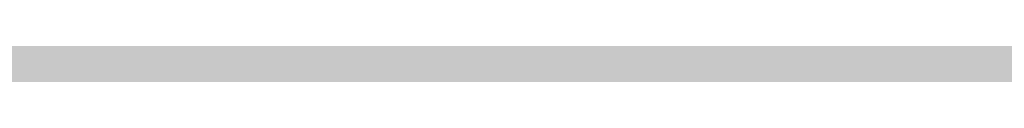
# Model space of a CAD drawing. Units: inches. Extents: x 2091 to 2899, y 967 to 2217.
# Tile 184 of 256: x 2203.16122 to 2203.18039, y 1152.24748 to 1152.2479. Entities that reach past the tile are written whole.
import ezdxf

# ---------------------------------------------------------------- set-up
doc = ezdxf.new("R2010")
doc.units = ezdxf.units.IN
doc.layers.add('A-WALL-PATT', color=141, linetype='Continuous', lineweight=13, true_color=0xadddf7)

msp = doc.modelspace()

# ---------------------------------------------------------------- hatches: boundary and pattern name
at = {"layer": 'A-WALL-PATT'}
h = msp.add_hatch(color=256, dxfattribs=at)
h.dxf.hatch_style = 1
h.paths.add_polyline_path([(2803.143603, 2050.919059), (2203.143603, 2050.919059), (2203.143603, 1090.919059), (2803.143603, 1090.919059)])
h.paths.add_polyline_path([(2635.79885, 1147.540465), (2674.524052, 1147.540465, 0.376086), (2678.529665, 1152.880202), (2678.529665, 1159.556473, 0.333335), (2674.524319, 1163.561846), (2674.524319, 1163.56185), (2674.524319, 1192.93439), (2635.805971, 1192.93439), (2597.087622, 1192.93439), (2597.087622, 1163.561846, 0.333335), (2593.082276, 1159.556473), (2593.082276, 1152.880202, 0.376086), (2597.087889, 1147.540465)], flags=0)
h.paths.add_polyline_path([(2436.010433, 1278.240778, 0.000483), (2435.952643, 1278.215027, -0.001328), (2435.935625, 1278.111693, -0.001711), (2436.11644, 1278.040758, 0.002185)], flags=0)
h.paths.add_polyline_path([(2794.143603, 1143.419059), (2794.143603, 1347.419059), (2543.370171, 1347.419059), (2543.370171, 1351.919059), (2794.143603, 1351.919059), (2794.143603, 1392.713555), (2793.947398, 1392.713555), (2793.947398, 1473.5369), (2794.143603, 1473.5369), (2794.143603, 1531.919059), (2650.143603, 1531.919059), (2650.143603, 1536.419059), (2794.143603, 1536.419059), (2794.143603, 1692.419059), (2609.375609, 1692.419059), (2609.375609, 1644.419059), (2604.875609, 1644.419059), (2604.875609, 1744.919059), (2609.375609, 1744.919059), (2609.375609, 1696.919059), (2794.143603, 1696.919059), (2794.143603, 1780.919059), (2609.643603, 1780.919059), (2493.875609, 1780.919059), (2493.875609, 1785.419059), (2609.643603, 1785.419059), (2794.143603, 1785.419059), (2794.143603, 1847.938821), (2793.951222, 1847.938821), (2793.951222, 1928.762166), (2794.143603, 1928.762166), (2794.143603, 1941.419059), (2614.143603, 1941.419059), (2614.143603, 1821.419059), (2609.643603, 1821.419059), (2609.643603, 1941.419059), (2392.143603, 1941.419059), (2392.143603, 1819.919059), (2387.643603, 1819.919059), (2387.643603, 1941.419059), (2212.143603, 1941.419059), (2212.143603, 1783.919059), (2392.143603, 1783.919059), (2392.143603, 1780.919059), (2212.143603, 1780.919059), (2212.143603, 1629.419059), (2387.643603, 1629.419059), (2387.643603, 1744.919059), (2392.143603, 1744.919059), (2392.143603, 1627.919059), (2317.143603, 1627.919059), (2317.143603, 1551.419059), (2317.143603, 1536.419059), (2459.383591, 1536.419059), (2459.383591, 1602.39648), (2463.883591, 1602.39648), (2463.883591, 1531.919059), (2456.643603, 1531.919059), (2456.643603, 1529.919059), (2452.143603, 1529.919059), (2452.143603, 1531.919059), (2312.643603, 1531.919059), (2312.643603, 1551.419059), (2306.143603, 1551.419059), (2306.143603, 1555.919059), (2308.143603, 1555.919059), (2308.143603, 1551.419059), (2312.643603, 1551.419059), (2312.643603, 1627.919059), (2212.143603, 1627.919059), (2212.143603, 1555.919059), (2270.143603, 1555.919059), (2270.143603, 1551.419059), (2212.143603, 1551.419059), (2212.143603, 1351.919059), (2272.143603, 1351.919059), (2272.143603, 1347.419059), (2212.143603, 1347.419059), (2212.143603, 1275.419059), (2308.143603, 1275.419059), (2308.143603, 1351.919059), (2452.143603, 1351.919059), (2452.143603, 1493.919059), (2456.643603, 1493.919059), (2456.643603, 1347.419059), (2312.643603, 1347.419059), (2312.643603, 1270.919059), (2212.143603, 1270.919059), (2212.143603, 1099.919059), (2281.237523, 1099.919059), (2282.871041, 1110.913803), (2282.008341, 1116.996603), (2278.557741, 1121.420403), (2268.205641, 1128.056203), (2272.087641, 1128.056203), (2273.812941, 1131.927003), (2279.420341, 1134.691903), (2285.027841, 1135.244903), (2287.615841, 1137.456803), (2288.047141, 1138.009803), (2289.341141, 1140.774703), (2291.066541, 1139.668703), (2292.360541, 1135.244903), (2295.379841, 1136.903803), (2296.242541, 1135.797903), (2297.105241, 1133.033003), (2300.124641, 1138.009803), (2303.143941, 1138.009803), (2304.437941, 1135.797903), (2303.143941, 1133.586003), (2306.594641, 1134.691903), (2307.888741, 1133.033003), (2310.908041, 1135.244903), (2313.927441, 1134.138903), (2315.62686, 1132.427102), (2308.320041, 1117.549603), (2290.203841, 1109.807903), (2288.909841, 1103.172103), (2289.272309, 1099.919059), (2434.918227, 1099.919059), (2431.593227, 1124.788059), (2429.930227, 1169.553059), (2430.927185, 1240.519694), (2435.658926, 1238.186126), (2437.135227, 1196.554059), (2438.798227, 1143.973059), (2442.678227, 1111.998059), (2446.558227, 1099.919059), (2794.143603, 1099.919059), (2794.143603, 1138.919059), (2548.032447, 1138.919059), (2548.032447, 1143.419059), (2548.032447, 1148.819059), (2546.668457, 1148.031559), (2528.685692, 1179.178622, 0.256256), (2512.032447, 1148.819059), (2512.032447, 1143.419059), (2512.032447, 1138.919059), (2507.532447, 1138.919059), (2507.532447, 1143.419059), (2507.532447, 1148.819059, 0.256256), (2490.879202, 1179.178622), (2472.896437, 1148.031559), (2471.532447, 1148.819059), (2471.532447, 1143.419059), (2467.032447, 1143.419059), (2467.032447, 1269.945786, 0.039061), (2460.909987, 1273.580059), (2467.032447, 1273.580059), (2467.032447, 1286.325364, 0.014511), (2465.216194, 1286.761905), (2467.032447, 1287.052576), (2467.032447, 1323.419059), (2471.532447, 1323.419059), (2471.532447, 1148.819059), (2489.532447, 1179.995973), (2490.896437, 1179.208473), (2490.879202, 1179.178622, -0.256256), (2507.532447, 1148.819059), (2507.532447, 1143.419059), (2512.032447, 1143.419059), (2512.032447, 1148.819059, -0.256256), (2528.685692, 1179.178622), (2528.668457, 1179.208473), (2530.032447, 1179.995973), (2548.032447, 1148.819059), (2548.032447, 1143.419059)], flags=16)
h.paths.add_polyline_path([(2607.768546, 1200.945083), (2607.768546, 1265.030625), (2597.087622, 1281.052011), (2619.784585, 1281.052011), (2627.795278, 1337.12686), (2635.79885, 1337.12686), (2643.816663, 1337.12686), (2651.827356, 1281.052011), (2674.524319, 1281.052011), (2663.843395, 1265.030625), (2663.843395, 1200.945083), (2635.805971, 1200.945083)], flags=0)
edge = h.paths.add_edge_path(flags=0)
edge.add_ellipse((13303.896215, 1272.998725), major_axis=(-10595.31304, 0.000001), ratio=0.842303870086, start_angle=0.6282372191, end_angle=0.6465540999, ccw=False)
edge.add_ellipse((2711.70045, 1156.852678), major_axis=(2.219769, 0), ratio=0.84230387, start_angle=111.535244, end_angle=180.628237, ccw=False)
edge.add_ellipse((13303.156292, 1272.998725), major_axis=(-10593.026306, 0), ratio=0.842303869544, start_angle=0.5282714718, end_angle=0.6465540971, ccw=False)
edge.add_line((2710.764596, 1175.333295), (2710.129986, 1175.333295))
edge.add_ellipse((2710.129986, 1176.579775), major_axis=(1.479846, 0), ratio=0.84230387, start_angle=180, end_angle=270, ccw=False)
edge.add_line((2708.65014, 1176.579775), (2708.65014, 1200.782914))
edge.add_ellipse((2710.129986, 1200.782914), major_axis=(1.479846, 0), ratio=0.84230387, start_angle=90, end_angle=180, ccw=False)
edge.add_line((2710.129986, 1202.029394), (2710.465075, 1202.029394))
edge.add_ellipse((13303.156292, 1272.998725), major_axis=(-10593.026306, 0), ratio=0.842303869544, start_angle=-0.0902290886, end_angle=0.3838667788, ccw=False)
edge.add_ellipse((2710.129986, 1290.927031), major_axis=(-1.479846, 0), ratio=0.84230387, start_angle=0, end_angle=90, ccw=False)
edge.add_line((2708.65014, 1290.927031), (2708.65014, 1315.13017))
edge.add_ellipse((2710.129986, 1315.13017), major_axis=(-1.479846, 0), ratio=0.84230387, start_angle=-90, end_angle=0, ccw=False)
edge.add_line((2710.129986, 1316.37665), (2710.706314, 1316.37665))
edge.add_ellipse((3238.40172, 1296.289566), major_axis=(528.234, 0), ratio=0.8423038695, start_angle=176.34957241, end_angle=177.82004969, ccw=False)
edge.add_ellipse((2775.063043, 1071.450696), major_axis=(313.307761, 0), ratio=0.8423038695, start_angle=102.12596555, end_angle=103.78052899, ccw=False)
edge.add_ellipse((2775.063043, 1078.305698), major_axis=(-305.302891, 0), ratio=0.8423038695, start_angle=-79.790461, end_angle=-77.55537271, ccw=False)
edge.add_ellipse((2695.141767, 1541.975383), major_axis=(-250.960216, 0), ratio=0.8423038695, start_angle=99.25656601, end_angle=102.55493264)
edge.add_line((2741.410326, 1334.214255), (2747.132545, 1337.378477))
edge.add_ellipse((2747.538616, 1336.857478), major_axis=(-0.739923, 0), ratio=0.8423039, start_angle=270, end_angle=307.93313, ccw=False)
edge.add_ellipse((2747.538616, 1336.857478), major_axis=(-0.739923, 0), ratio=0.8423039, start_angle=232.06687, end_angle=270, ccw=False)
edge.add_line((2747.944687, 1337.378477), (2753.666906, 1334.214255))
edge.add_ellipse((2799.935466, 1541.975383), major_axis=(250.960216, 0), ratio=0.8423038695, start_angle=257.44506736, end_angle=260.74343399)
edge.add_ellipse((2720.014189, 1078.305698), major_axis=(305.302891, 0), ratio=0.8423038695, start_angle=77.55537271, end_angle=79.790461, ccw=False)
edge.add_ellipse((2720.014189, 1071.450696), major_axis=(-313.307761, 0), ratio=0.8423038695, start_angle=256.21947101, end_angle=257.87403445, ccw=False)
edge.add_ellipse((2256.675512, 1296.289566), major_axis=(-528.234, 0), ratio=0.8423038695, start_angle=182.17995031, end_angle=183.65042759, ccw=False)
edge.add_line((2784.370918, 1316.37665), (2784.947247, 1316.37665))
edge.add_ellipse((2784.947247, 1315.13017), major_axis=(1.479846, 0), ratio=0.84230387, start_angle=0, end_angle=90, ccw=False)
edge.add_line((2786.427093, 1315.13017), (2786.427093, 1290.927031))
edge.add_ellipse((2784.947247, 1290.927031), major_axis=(1.479846, 0), ratio=0.84230387, start_angle=270, end_angle=360, ccw=False)
edge.add_ellipse((-7808.07906, 1272.998725), major_axis=(10593.026306, 0), ratio=0.842303869544, start_angle=-0.3838667788, end_angle=0.0902290886, ccw=False)
edge.add_line((2784.612157, 1202.029394), (2784.947247, 1202.029394))
edge.add_ellipse((2784.947247, 1200.782914), major_axis=(1.479846, 0), ratio=0.84230387, start_angle=0, end_angle=90, ccw=False)
edge.add_line((2786.427093, 1200.782914), (2786.427093, 1176.579775))
edge.add_ellipse((2784.947247, 1176.579775), major_axis=(-1.479846, 0), ratio=0.84230387, start_angle=90, end_angle=180, ccw=False)
edge.add_line((2784.947247, 1175.333295), (2784.312636, 1175.333295))
edge.add_ellipse((-7808.07906, 1272.998725), major_axis=(10593.026306, 0), ratio=0.842303869544, start_angle=-0.6186431963, end_angle=-0.5282714718, ccw=False)
edge.add_ellipse((2783.376783, 1156.852678), major_axis=(-2.219769, 0), ratio=0.84230387, start_angle=179.371763, end_angle=248.464757, ccw=False)
edge.add_ellipse((-7808.818983, 1272.998725), major_axis=(-10595.31304, 0.000004), ratio=0.842303865762, start_angle=179.3534459226, end_angle=179.3717628034, ccw=False)
edge.add_ellipse((2780.297303, 1153.500793), major_axis=(-5.246426, 0), ratio=0.84230387, start_angle=90, end_angle=179.353446, ccw=False)
edge.add_line((2780.297303, 1149.081708), (2714.77993, 1149.081708))
edge.add_ellipse((2714.77993, 1153.500793), major_axis=(5.246426, 0), ratio=0.84230387, start_angle=180.646554, end_angle=270, ccw=False)
edge = h.paths.add_edge_path(flags=0)
edge.add_line((2718.187367, 1151.007833), (2718.187367, 1170.472364))
edge.add_ellipse((2721.14706, 1170.472364), major_axis=(-2.959692, 0), ratio=0.84230387, start_angle=-90, end_angle=0, ccw=False)
edge.add_line((2721.14706, 1172.965324), (2773.930173, 1172.965324))
edge.add_ellipse((2773.930173, 1170.472364), major_axis=(-2.959692, 0), ratio=0.84230387, start_angle=180, end_angle=270, ccw=False)
edge.add_line((2776.889865, 1170.472364), (2776.889865, 1151.007833))
edge.add_line((2776.889865, 1151.007833), (2718.187367, 1151.007833))
edge = h.paths.add_edge_path(flags=0)
edge.add_line((2718.187367, 1180.23415), (2718.187367, 1199.057834))
edge.add_ellipse((2747.538616, 1320.39864), major_axis=(147.017924, 0), ratio=0.8423038695, start_angle=256.40186531, end_angle=283.59813469)
edge.add_line((2776.889865, 1199.057834), (2776.889865, 1180.23415))
edge.add_ellipse((2747.538616, 1301.574956), major_axis=(147.017924, 0), ratio=0.8423038695, start_angle=256.40186531, end_angle=283.59813469, ccw=False)
edge = h.paths.add_edge_path(flags=0)
edge.add_ellipse((13303.156292, 1272.998725), major_axis=(-10591.54646, 0), ratio=0.842303869555, start_angle=0.0555943135, end_angle=0.3777641939, ccw=False)
edge.add_line((2711.616859, 1262.72171), (2715.667408, 1249.495396))
edge.add_ellipse((6413.891963, 1241.691919), major_axis=(-3698.236159, 0), ratio=0.84230386955, start_angle=-0.120897369, end_angle=0.364076349)
edge.add_line((2715.761038, 1218.192455), (2711.934307, 1203.167361))
edge = h.paths.add_edge_path(flags=0)
edge.add_line((2718.187367, 1251.074566), (2716.002485, 1267.450435))
edge.add_ellipse((2742.151175, 1202.18954), major_axis=(81.772585, 0), ratio=0.84230387, start_angle=94.27742096, end_angle=111.8349538, ccw=False)
edge.add_line((2737.009748, 1270.930626), (2758.067484, 1270.930626))
edge.add_ellipse((2752.926058, 1202.18954), major_axis=(81.772585, 0), ratio=0.84230387, start_angle=68.1650462, end_angle=85.72257904, ccw=False)
edge.add_line((2779.074747, 1267.450435), (2776.889865, 1251.074566))
edge.add_ellipse((2750.338059, 1187.885356), major_axis=(79.579664, 0), ratio=0.84230387, start_angle=67.20808512, end_angle=85.1299304)
edge.add_line((2756.034656, 1254.743656), (2739.042576, 1254.743656))
edge.add_ellipse((2744.739174, 1187.885356), major_axis=(79.579664, 0), ratio=0.84230387, start_angle=94.8700696, end_angle=112.79191488)
edge = h.paths.add_edge_path(flags=0)
edge.add_line((2783.142926, 1203.167361), (2779.316194, 1218.192455))
edge.add_ellipse((-918.81473, 1241.691919), major_axis=(3698.236159, 0), ratio=0.84230386955, start_angle=-0.364076349, end_angle=0.120897369)
edge.add_line((2779.409825, 1249.495396), (2783.460373, 1262.72171))
edge.add_ellipse((-7808.07906, 1272.998725), major_axis=(-10591.54646, 0), ratio=0.84230386954, start_angle=179.6222358061, end_angle=179.9444056865, ccw=False)
edge = h.paths.add_edge_path(flags=0)
edge.add_ellipse((2734.200892, 1286.69044), major_axis=(-0.356609, 6.340078), ratio=0.60383358, start_angle=89.0020143, end_angle=253.657408, ccw=False)
edge.add_line((2730.369001, 1286.541806), (2730.369001, 1301.35198))
edge.add_line((2730.369001, 1301.35198), (2735.913311, 1305.214803))
edge.add_ellipse((2736.384917, 1304.734561), major_axis=(0.739923, 0), ratio=0.8423039, start_angle=90, end_angle=134.480211, ccw=False)
edge.add_line((2736.384917, 1305.357801), (2738.032783, 1305.357801))
edge.add_line((2738.032783, 1305.357801), (2738.032783, 1307.707927))
edge.add_ellipse((2794.201642, 1307.707927), major_axis=(56.168859, 0), ratio=0.84230387, start_angle=150.5614304, end_angle=180, ccw=False)
edge.add_ellipse((2700.875591, 1307.707927), major_axis=(-56.168859, 0), ratio=0.84230387, start_angle=180, end_angle=209.4385696, ccw=False)
edge.add_line((2757.04445, 1307.707927), (2757.04445, 1305.357801))
edge.add_line((2757.04445, 1305.357801), (2758.692316, 1305.357801))
edge.add_ellipse((2758.692316, 1304.734561), major_axis=(-0.739923, 0), ratio=0.8423039, start_angle=225.519789, end_angle=270, ccw=False)
edge.add_line((2759.163922, 1305.214803), (2764.708231, 1301.35198))
edge.add_line((2764.708231, 1301.35198), (2764.708231, 1286.541806))
edge.add_ellipse((2760.87634, 1286.69044), major_axis=(0.356609, 6.340078), ratio=0.60383358, start_angle=106.342592, end_angle=270.9979857, ccw=False)
edge.add_line((2757.04445, 1285.79709), (2757.04445, 1307.707927))
edge.add_ellipse((2700.875591, 1307.707927), major_axis=(-56.168859, 0), ratio=0.84230387, start_angle=180, end_angle=209.4385696)
edge.add_ellipse((2794.201642, 1307.707927), major_axis=(56.168859, 0), ratio=0.84230387, start_angle=150.5614304, end_angle=180)
edge.add_line((2738.032783, 1307.707927), (2738.032783, 1285.79709))
h.paths.add_polyline_path([(2417.812273, 1104.449704), (2413.492273, 1102.529704), (2410.612273, 1103.969704), (2409.172273, 1106.369704), (2407.252273, 1107.329704), (2406.292273, 1109.729704), (2405.332273, 1114.049704), (2405.332273, 1117.889704), (2406.292273, 1120.129704), (2407.252273, 1119.809704), (2408.848322, 1118.327658), (2410.173945, 1119.42417), (2410.211273, 1120.405704), (2411.040731, 1121.419054), (2410.699273, 1119.858704), (2410.173945, 1119.42417), (2410.088452, 1117.176109), (2411.132836, 1116.206324), (2413.972273, 1119.329704), (2416.852273, 1120.769704), (2416.869721, 1120.798784), (2417.035071, 1119.405116), (2417.896213, 1118.143384), (2418.292273, 1118.369704), (2419.544447, 1120.039269), (2419.360915, 1118.387487), (2419.032108, 1119.356151), (2418.398939, 1118.511926), (2419.252273, 1114.529704), (2418.794091, 1107.198795)], flags=0)
h.paths.add_polyline_path([(2508.870171, 1347.419059), (2508.370171, 1347.419059), (2508.370171, 1351.919059), (2508.870171, 1351.919059)], flags=0)
h.paths.add_polyline_path([(2473.370171, 1347.419059), (2472.370171, 1347.419059), (2467.870171, 1347.419059), (2467.870171, 1455.419059), (2472.370171, 1455.419059), (2472.370171, 1352.419059), (2473.370171, 1352.419059)], flags=0)
h.paths.add_polyline_path([(2352.106244, 1217.446197), (2349.226244, 1218.886197), (2347.786244, 1221.286197), (2345.866244, 1222.246197), (2344.906244, 1224.646197), (2343.946244, 1228.966197), (2343.946244, 1232.806197), (2344.906244, 1235.046197), (2345.866244, 1234.726197), (2347.462293, 1233.244152), (2348.787916, 1234.340663), (2348.825244, 1235.322197), (2349.654702, 1236.335547), (2349.313244, 1234.775197), (2348.787916, 1234.340663), (2348.702423, 1232.092603), (2349.746807, 1231.122817), (2352.586244, 1234.246197), (2355.466244, 1235.686197), (2355.483692, 1235.715277), (2355.649043, 1234.321609), (2356.510185, 1233.059877), (2356.906244, 1233.286197), (2358.158418, 1234.955762), (2357.974887, 1233.30398), (2357.646079, 1234.272644), (2357.012911, 1233.428419), (2357.866244, 1229.446197), (2357.408062, 1222.115288), (2356.426244, 1219.366197)], flags=0)
h.paths.add_polyline_path([(2348.2968, 1112.22442), (2347.0138, 1112.31042), (2345.5298, 1114.12742), (2345.7318, 1115.85842), (2346.8118, 1116.98242), (2346.8118, 1114.64642), (2345.8668, 1114.21442), (2346.8798, 1114.30042)], flags=0)
h.paths.add_polyline_path([(2347.0138, 1110.92642), (2346.2718, 1110.49342), (2346.6098, 1111.18642)], flags=0)
h.paths.add_polyline_path([(2345.8668, 1118.19442), (2345.5298, 1117.32942), (2343.7078, 1118.02142), (2344.3828, 1118.62642)], flags=0)
h.paths.add_polyline_path([(2346.6768, 1109.28242), (2346.0698, 1108.07142), (2345.8668, 1110.06142)], flags=0)
h.paths.add_polyline_path([(2345.0568, 1119.75142), (2343.6398, 1119.75142), (2343.9778, 1121.13542)], flags=0)
h.paths.add_polyline_path([(2345.2598, 1116.55042), (2345.1248, 1115.85842), (2344.9218, 1115.68542), (2344.7198, 1116.37742)], flags=0)
h.paths.add_polyline_path([(2345.6648, 1112.31042), (2345.4618, 1111.53242), (2344.0448, 1111.96442), (2344.6518, 1112.57042)], flags=0)
h.paths.add_polyline_path([(2345.1918, 1113.34942), (2344.4498, 1113.86842), (2344.7198, 1114.38742)], flags=0)
h.paths.add_polyline_path([(2344.6518, 1116.80942), (2344.1798, 1115.68542), (2344.6518, 1115.33942), (2343.9098, 1114.90642), (2343.0328, 1115.94442), (2343.6398, 1116.46342)], flags=0)
h.paths.add_polyline_path([(2345.8668, 1106.68642), (2344.9898, 1105.56242), (2344.5168, 1106.60042)], flags=0)
h.paths.add_polyline_path([(2344.8548, 1110.06142), (2344.5168, 1109.28242), (2344.1128, 1109.71542)], flags=0)
h.paths.add_polyline_path([(2344.0448, 1113.52242), (2343.4378, 1113.08942), (2342.7628, 1113.95442)], flags=0)
h.paths.add_polyline_path([(2344.3148, 1111.01242), (2342.9648, 1110.32042), (2342.9648, 1111.09942)], flags=0)
h.paths.add_polyline_path([(2345.1248, 1104.69742), (2344.5848, 1103.74542), (2344.4498, 1104.26442)], flags=0)
h.paths.add_polyline_path([(2342.8298, 1121.22242), (2341.7498, 1120.53042), (2340.5358, 1121.04942), (2340.1308, 1121.82842), (2340.6708, 1122.95242), (2341.1428, 1121.82842), (2341.6148, 1122.00142)], flags=0)
h.paths.add_polyline_path([(2342.9648, 1119.75142), (2343.0328, 1118.45342), (2342.0878, 1118.02142), (2342.0198, 1119.49142)], flags=0)
h.paths.add_polyline_path([(2342.6948, 1116.89642), (2341.9528, 1116.63642), (2342.0198, 1117.32942)], flags=0)
h.paths.add_polyline_path([(2343.0328, 1112.22442), (2342.0198, 1111.79142), (2341.5478, 1112.22442), (2342.3578, 1113.34942)], flags=0)
h.paths.add_polyline_path([(2343.7748, 1104.43742), (2342.6278, 1102.88042), (2342.6948, 1104.61042), (2343.4378, 1105.12942)], flags=0)
h.paths.add_polyline_path([(2342.0198, 1115.07942), (2340.8058, 1115.51242), (2340.9408, 1116.37742)], flags=0)
h.paths.add_polyline_path([(2341.4808, 1120.09742), (2341.4808, 1119.40542), (2341.0758, 1119.57842), (2341.1428, 1120.09742)], flags=0)
h.paths.add_polyline_path([(2341.8178, 1114.47342), (2340.9408, 1113.08942), (2340.8058, 1114.56042)], flags=0)
h.paths.add_polyline_path([(2341.1428, 1118.54042), (2340.9408, 1116.98242), (2339.0508, 1117.67542), (2339.0508, 1118.62642)], flags=0)
h.paths.add_polyline_path([(2342.6948, 1101.66842), (2341.9528, 1101.84142), (2342.5598, 1102.36142)], flags=0)
h.paths.add_polyline_path([(2340.3328, 1119.66542), (2338.4438, 1119.57842), (2337.9038, 1120.35742), (2339.6578, 1120.61642)], flags=0)
h.paths.add_polyline_path([(2340.3328, 1115.33942), (2340.0628, 1113.69542), (2339.3878, 1115.33942)], flags=0)
h.paths.add_polyline_path([(2341.8178, 1103.83142), (2341.5478, 1102.88042), (2341.1428, 1103.65842)], flags=0)
h.paths.add_polyline_path([(2339.0508, 1122.86642), (2337.2958, 1121.82842), (2337.0938, 1123.12542), (2337.7688, 1123.81842)], flags=0)
h.paths.add_polyline_path([(2339.1178, 1121.74142), (2338.8478, 1121.22242), (2338.1738, 1121.04942), (2338.3758, 1121.56842)], flags=0)
h.paths.add_polyline_path([(2339.1858, 1119.31942), (2338.6458, 1118.71342), (2338.2408, 1118.10742), (2338.2408, 1118.88642)], flags=0)
h.paths.add_polyline_path([(2341.1428, 1101.92842), (2340.6028, 1101.23642), (2340.0628, 1101.84142), (2340.6028, 1102.36142)], flags=0)
h.paths.add_polyline_path([(2337.6338, 1117.76142), (2336.6208, 1118.28042), (2337.2958, 1118.97242)], flags=0)
h.paths.add_polyline_path([(2336.8238, 1119.57842), (2334.7988, 1118.97242), (2335.2038, 1120.35742), (2336.5538, 1120.87642)], flags=0)
h.paths.add_polyline_path([(2339.1178, 1100.45742), (2337.3638, 1100.54342), (2336.7558, 1101.23642)], flags=0)
h.paths.add_polyline_path([(2336.3508, 1122.43342), (2336.0138, 1121.91442), (2334.9338, 1122.43342), (2334.5288, 1123.47142), (2335.7438, 1122.77942)], flags=0)
h.paths.add_polyline_path([(2334.7318, 1120.87642), (2334.2588, 1120.35742), (2334.0568, 1120.78942), (2334.5968, 1121.30842)], flags=0)
h.paths.add_polyline_path([(2334.4618, 1122.17442), (2332.5718, 1121.30842), (2331.3568, 1122.17442), (2332.0998, 1122.86642)], flags=0)
h.paths.add_polyline_path([(2334.2588, 1118.54042), (2333.3818, 1118.45342), (2333.6518, 1119.31942)], flags=0)
h.paths.add_polyline_path([(2335.5418, 1102.27442), (2334.1918, 1102.62042), (2335.2718, 1103.31242)], flags=0)
h.paths.add_polyline_path([(2332.7068, 1119.66542), (2331.6948, 1120.44342), (2332.5048, 1120.78942)], flags=0)
h.paths.add_polyline_path([(2334.7318, 1101.14942), (2333.5168, 1101.58242), (2333.9888, 1101.75542)], flags=0)
h.paths.add_polyline_path([(2332.6398, 1116.63642), (2331.0868, 1116.29042), (2331.9648, 1118.19442)], flags=0)
h.paths.add_polyline_path([(2330.7498, 1121.56842), (2330.2768, 1120.27042), (2328.5228, 1119.31942), (2328.9948, 1121.04942)], flags=0)
h.paths.add_polyline_path([(2330.7498, 1118.62642), (2330.0078, 1117.50242), (2329.8728, 1118.02142)], flags=0)
h.paths.add_polyline_path([(2332.0998, 1102.36142), (2330.5468, 1102.01442), (2331.6948, 1102.96642)], flags=0)
h.paths.add_polyline_path([(2329.5348, 1113.60842), (2329.0628, 1112.31042), (2328.5898, 1113.34942)], flags=0)
h.paths.add_polyline_path([(2328.3878, 1117.84842), (2327.5098, 1116.55042), (2327.1728, 1117.76142)], flags=0)
h.paths.add_polyline_path([(2329.7378, 1106.51342), (2329.5348, 1105.30242), (2328.2528, 1106.08142)], flags=0)
h.paths.add_polyline_path([(2328.6578, 1114.38742), (2328.0498, 1114.12742), (2328.3198, 1114.90642)], flags=0)
h.paths.add_polyline_path([(2328.3198, 1112.22442), (2327.1058, 1112.13742), (2326.7008, 1112.65642)], flags=0)
h.paths.add_polyline_path([(2326.9028, 1115.25242), (2326.7008, 1114.12742), (2325.2158, 1113.60842), (2326.0928, 1115.33942)], flags=0)
h.paths.add_polyline_path([(2326.6328, 1108.33042), (2326.0928, 1107.37942), (2325.8908, 1108.50342), (2326.4978, 1109.10942)], flags=0)
h.paths.add_polyline_path([(2615.143603, 1531.919059), (2609.643603, 1531.919059), (2609.643603, 1620.419059), (2614.143603, 1620.419059), (2614.143603, 1536.419059), (2615.143603, 1536.419059)], flags=0)
h.paths.add_polyline_path([(2545.143603, 1563.419059), (2464.143603, 1563.419059), (2464.143603, 1632.419059), (2509.143603, 1632.419059), (2509.143603, 1627.919059), (2509.143603, 1603.919059), (2468.643603, 1603.919059), (2468.643603, 1567.919059), (2540.643603, 1567.919059), (2540.643603, 1591.919059), (2545.143603, 1591.919059)], flags=0)
h.paths.add_polyline_path([(2388.969048, 1549.985735), (2357.434181, 1549.985735), (2357.434181, 1623.360778), (2399.362777, 1623.360778), (2435.689465, 1623.360778), (2435.592547, 1602.559273), (2435.592547, 1602.39648), (2388.969048, 1602.39648)], flags=0)
h.paths.add_polyline_path([(2388.880628, 1555.809151), (2374.904429, 1555.809151), (2374.904429, 1600.571564), (2374.904429, 1615.457645), (2406.350877, 1615.457645), (2406.350877, 1618.939431), (2412.174293, 1615.457645), (2406.350877, 1611.97586), (2406.350877, 1615.457645), (2388.880628, 1615.457645)], flags=0)
h.paths.add_polyline_path([(2568.875609, 1644.419059), (2453.375609, 1644.419059), (2453.375609, 1785.419059), (2457.875609, 1785.419059), (2457.875609, 1648.919059), (2568.875609, 1648.919059)], flags=0)
h.paths.add_polyline_path([(2212.143603, 1945.919059), (2212.143603, 2041.919059), (2794.143603, 2041.919059), (2794.143603, 1945.919059)], flags=16)
h.paths.add_polyline_path([(2271.082728, 1964.317238), (2776.852968, 1964.317238), (2776.852968, 2037.169623), (2271.082728, 2037.169623)], flags=8)
h.paths.add_polyline_path([(2380.649285, 1536.824144), (2461.040809, 1536.824144), (2461.040809, 1554.652587), (2380.649285, 1554.652587)], flags=8)
h.paths.add_polyline_path([(2240.755709, 1609.725451), (2309.185829, 1609.725451), (2309.185829, 1617.698204), (2240.755709, 1617.698204)], flags=8)
h.paths.add_polyline_path([(2212.677255, 1313.504102), (2282.59152, 1313.504102), (2282.59152, 1322.745239), (2212.677255, 1322.745239)], flags=8)
h.paths.add_polyline_path([(2457.111976, 1114.778574), (2558.481581, 1114.778574), (2558.481581, 1142.219682), (2457.111976, 1142.219682)], flags=8)
h.paths.add_polyline_path([(2473.442337, 1273.010067), (2604.641226, 1273.010067), (2604.641226, 1318.346935), (2473.442337, 1318.346935)], flags=8)
h.paths.add_polyline_path([(2638.876302, 1626.977432), (2684.250367, 1627.976738), (2684.038483, 1637.597494), (2638.664417, 1636.598188)], flags=8)
h.paths.add_polyline_path([(2537.590554, 1453.793447), (2628.389547, 1453.793447), (2628.389547, 1475.344811), (2537.590554, 1475.344811)], flags=8)
h.paths.add_polyline_path([(2504.137638, 1714.632397), (2554.647187, 1714.632397), (2554.647187, 1730.237712), (2504.137638, 1730.237712)], flags=8)
h.paths.add_polyline_path([(2487.501181, 1575.651872), (2535.097121, 1575.651872), (2535.097121, 1598.377646), (2487.501181, 1598.377646)], flags=8)
h.paths.add_polyline_path([(2709.0994, 1735.710278), (2740.016601, 1735.710278), (2740.016601, 1749.937641), (2709.0994, 1749.937641)], flags=8)
h.paths.add_polyline_path([(2442.438424, 1792.171657), (2564.728835, 1792.171657), (2564.728835, 1842.000163), (2442.438424, 1842.000163)], flags=8)
h.paths.add_polyline_path([(2655.815801, 1809.644076), (2789.520142, 1806.693796), (2790.084977, 1832.291638), (2656.380635, 1835.241918)], flags=8)
h.paths.add_polyline_path([(2234.842697, 1797.720143), (2368.592851, 1794.768852), (2369.160718, 1820.504132), (2235.410564, 1823.455423)], flags=8)
h.paths.add_polyline_path([(2245.138466, 1644.006335), (2398.427733, 1640.6239), (2398.994842, 1666.32482), (2245.705575, 1669.707255)], flags=8)
h.paths.add_polyline_path([(2306.142847, 1431.168519), (2413.768314, 1428.793687), (2414.333148, 1454.391529), (2306.707682, 1456.76636)], flags=8)
h.paths.add_polyline_path([(2306.834582, 1458.233145), (2393.380484, 1456.323449), (2393.932808, 1481.354358), (2307.386907, 1483.264054)], flags=8)

doc.saveas('drawing.dxf')
